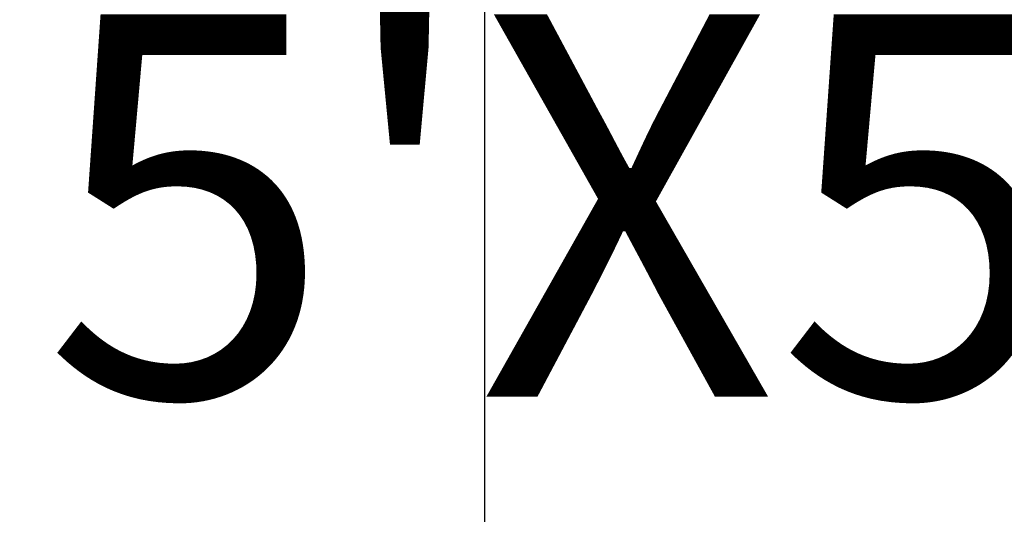
# Model space of a CAD drawing. Units: inches. Extents: x 2696 to 3240, y 1564 to 2310.
# Tile 34 of 76: x 3138 to 3161, y 1710 to 1722. Entities that reach past the tile are written whole.
import ezdxf

# ---------------------------------------------------------------- set-up
doc = ezdxf.new("R2010")
doc.units = ezdxf.units.IN
doc.layers.add('A-ANNO-DIMS', color=3, linetype='Continuous', lineweight=18)
doc.layers.add('A-AREA-IDEN', color=7, linetype='Continuous', lineweight=18)
doc.styles.add('TIMES NEW', font='times.ttf')
doc.styles.add('YQ_DIM', font='SUPEROS.SHX', dxfattribs={"width": 0.8, "bigfont": 'HZDX.SHX'})
doc.dimstyles.new('Siddhuu', dxfattribs={"dimtxt": 6, "dimasz": 2.5, "dimexe": 1.25, "dimexo": 0.625, "dimtad": 1, "dimdec": 1, "dimlunit": 4, "dimtxsty": 'TIMES NEW', "dimcen": 2.5, "dimclrd": 256, "dimclre": 1, "dimclrt": 7, "dimadec": 0, "dimazin": 0, "dimtfac": 1, "dimtdec": 1, "dimtmove": 0, "dimatfit": 3, "dimfxl": 1, "dimtolj": 1, "dimlwd": -1, "dimarcsym": 0})

# ---------------------------------------------------------------- blocks, each defined once
blk = doc.blocks.new('*D51')
at = {"layer": 'A-ANNO-DIMS', "color": 1, "lineweight": -2, "transparency": 16777216}
for p, q in [((3016.611, 1979.576), (3016.611, 1568.951)), ((3148.611, 1979.576), (3148.611, 1568.951))]:
    blk.add_line(p, q, dxfattribs=at)
at = {"layer": 'A-ANNO-DIMS', "transparency": 16777216}
blk.add_line((3019.111, 1570.201), (3146.111, 1570.201), dxfattribs=at)
for points in [[(3019.111, 1570.618), (3019.111, 1569.784), (3016.611, 1570.201)], [(3146.111, 1570.618), (3146.111, 1569.784), (3148.611, 1570.201)]]:
    blk.add_solid(points, dxfattribs=at)
at = {"layer": 'Defpoints', "color": 0, "transparency": 16777216}
for p in [(3016.611, 1980.201), (3148.611, 1980.201), (3148.611, 1570.201)]:
    blk.add_point(p, dxfattribs=at)
at = {"layer": 'A-ANNO-DIMS', "color": 7, "transparency": 16777216, "insert": (3082.611, 1573.878), "char_height": 6, "attachment_point": 5, "style": 'TIMES NEW'}
blk.add_mtext('\\A1;11\'-0"', dxfattribs=at)
blk = doc.blocks.new('*D52')
at = {"layer": 'A-ANNO-DIMS', "color": 1, "lineweight": -2, "transparency": 16777216}
for p, q in [((3148.611, 1979.576), (3148.611, 1568.951)), ((3190.611, 1979.576), (3190.611, 1568.951))]:
    blk.add_line(p, q, dxfattribs=at)
at = {"layer": 'A-ANNO-DIMS', "transparency": 16777216}
blk.add_line((3151.111, 1570.201), (3188.111, 1570.201), dxfattribs=at)
for points in [[(3151.111, 1570.618), (3151.111, 1569.784), (3148.611, 1570.201)], [(3188.111, 1570.618), (3188.111, 1569.784), (3190.611, 1570.201)]]:
    blk.add_solid(points, dxfattribs=at)
at = {"layer": 'Defpoints', "color": 0, "transparency": 16777216}
for p in [(3148.611, 1980.201), (3190.611, 1980.201), (3190.611, 1570.201)]:
    blk.add_point(p, dxfattribs=at)
at = {"layer": 'A-ANNO-DIMS', "color": 7, "transparency": 16777216, "insert": (3169.611, 1573.878), "char_height": 6, "attachment_point": 5, "style": 'TIMES NEW'}
blk.add_mtext('\\A1;3\'-6"', dxfattribs=at)
blk = doc.blocks.new('*D56')
at = {"layer": 'A-ANNO-DIMS', "color": 1, "lineweight": -2, "transparency": 16777216}
for p, q in [((2966.334, 1884.201), (3235.861, 1884.201)), ((2966.334, 1665.201), (3235.861, 1665.201))]:
    blk.add_line(p, q, dxfattribs=at)
at = {"layer": 'A-ANNO-DIMS', "transparency": 16777216}
blk.add_line((3234.611, 1667.701), (3234.611, 1881.701), dxfattribs=at)
for points in [[(3234.195, 1881.701), (3235.028, 1881.701), (3234.611, 1884.201)], [(3234.195, 1667.701), (3235.028, 1667.701), (3234.611, 1665.201)]]:
    blk.add_solid(points, dxfattribs=at)
at = {"layer": 'Defpoints', "color": 0, "transparency": 16777216}
for p in [(2965.709, 1884.201), (3234.611, 1884.201), (2965.709, 1665.201)]:
    blk.add_point(p, dxfattribs=at)
at = {"layer": 'A-ANNO-DIMS', "color": 7, "transparency": 16777216, "insert": (3230.934, 1774.701), "char_height": 6, "attachment_point": 5, "rotation": 90, "style": 'TIMES NEW'}
blk.add_mtext('\\A1;18\'-3"', dxfattribs=at)

msp = doc.modelspace()

# ---------------------------------------------------------------- texts
at = {"layer": 'A-AREA-IDEN', "insert": (3138.221, 1737.206), "char_height": 9, "attachment_point": 1, "style": 'YQ_DIM'}
msp.add_mtext_dynamic_manual_height_columns('TOILET\\P5\'X5\'4.5"', width=48.00324, gutter_width=12.5, heights=[0], dxfattribs=at)

# ---------------------------------------------------------------- dimensions: what is measured, and where the dimension line sits
at = {"layer": 'A-ANNO-DIMS'}
for base, p1, p2, picture, middle in [((3148.611, 1570.201), (3016.611, 1980.201), (3148.611, 1980.201), '*D51', (3082.611, 1573.878)), ((3190.611, 1570.201), (3148.611, 1980.201), (3190.611, 1980.201), '*D52', (3169.611, 1573.878))]:
    dim = msp.add_linear_dim(base=base, p1=p1, p2=p2, dimstyle='Siddhuu', override={"dimdec": 1, "dimlfac": 1, "dimrnd": 0, "dimzin": 1, "dimdsep": 46, "dimlunit": 4, "dimfrac": 2}, dxfattribs=at)
    dim.commit()
    dim.dimension.update_dxf_attribs({"geometry": picture, "text_midpoint": middle})
dim = msp.add_linear_dim(base=(3234.611, 1884.201), p1=(2965.709, 1665.201), p2=(2965.709, 1884.201), angle=90, dimstyle='Siddhuu', override={"dimdec": 1, "dimlfac": 1, "dimrnd": 0, "dimzin": 1, "dimdsep": 46, "dimlunit": 4, "dimfrac": 2}, dxfattribs=at)
dim.commit()
dim.dimension.update_dxf_attribs({"geometry": '*D56', "text_midpoint": (3230.934, 1774.701)})

doc.saveas('drawing.dxf')
